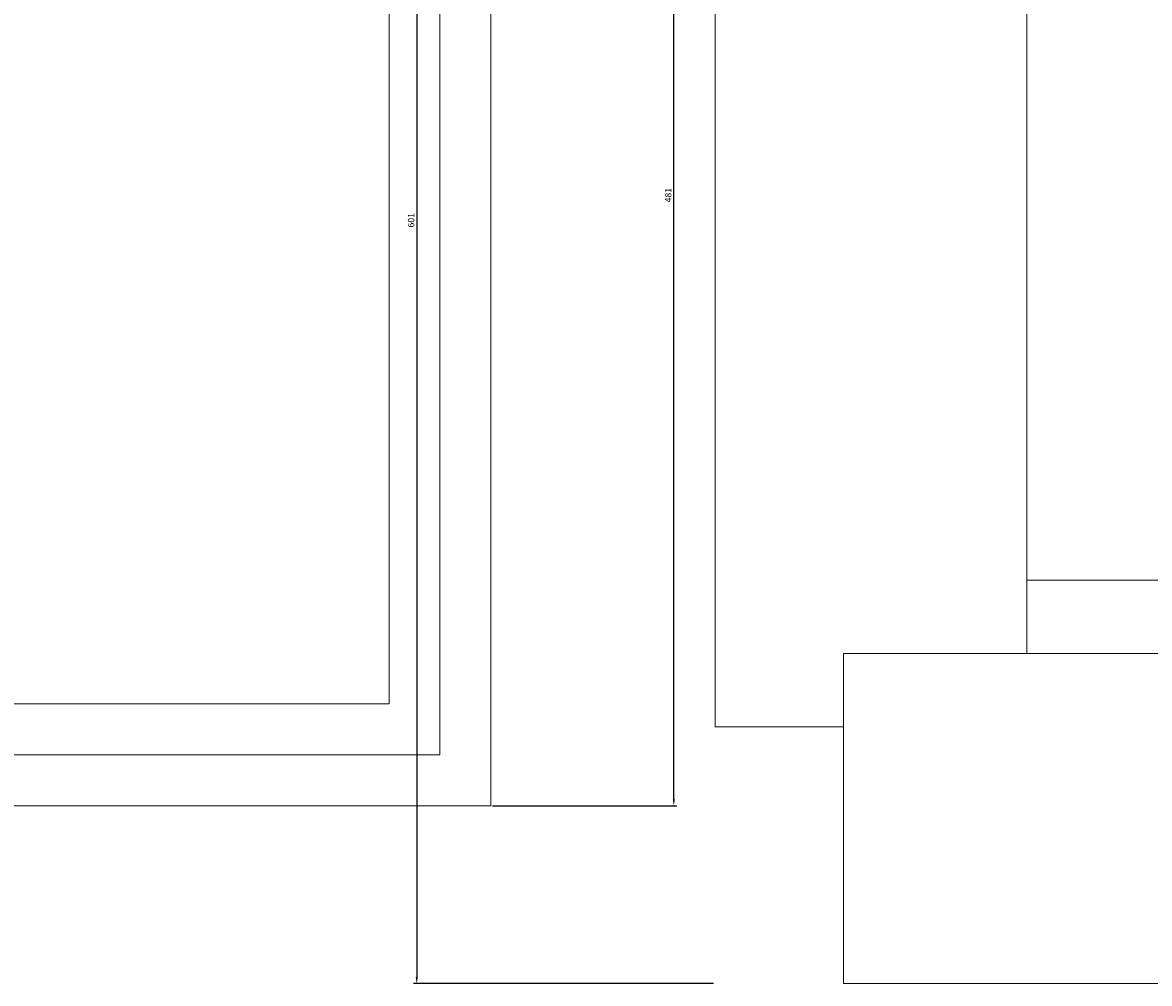
# Model space of a CAD drawing. Units: millimetres. Extents: x -857 to 54106, y -13666 to 13947.
# Tile 6 of 41: x 7861 to 8305, y 6233 to 6612. Entities that reach past the tile are written whole.
import ezdxf

# ---------------------------------------------------------------- set-up
doc = ezdxf.new("R2010")
doc.units = ezdxf.units.MM
for name, color, linetype, lineweight in [('A-ANNO-DIMS', 2, 'Continuous', 18), ('A-FURN', 21, 'Continuous', 18), ('A-FURNITURE', 25, 'Continuous', 9)]:
    doc.layers.add(name, color=color, linetype=linetype, lineweight=lineweight)
doc.styles.get("Standard").update_dxf_attribs({"font": 'arial.ttf'})
doc.dimstyles.new('ISO-25', dxfattribs={"dimtxt": 2.5, "dimasz": 2.5, "dimexe": 1.25, "dimexo": 0.625, "dimtad": 1, "dimtxsty": 'Standard', "dimcen": 2.5, "dimadec": 0, "dimazin": 0, "dimtfac": 1, "dimtmove": 0, "dimatfit": 3, "dimfxl": 1, "dimarcsym": 0})

# ---------------------------------------------------------------- blocks, each defined once
blk = doc.blocks.new('A$C21FE29A1')
at = {"layer": 'A-FURNITURE'}
for points in [[(0, 0), (24, 0), (24, 24), (0, 24)], [(1, 1), (23, 1), (23, 23), (1, 23)], [(2, 2), (22, 2), (22, 22), (2, 22)]]:
    blk.add_lwpolyline(points, close=True, dxfattribs=at)
blk = doc.blocks.new('A$C47E27A62')
at = {"layer": 'A-FURNITURE'}
for p, q in [((17.041, 0), (-17.041, 0)), ((17.041, 0), (17.041, -6.486)), ((17.041, -5.045), (19.563, -5.045)), ((19.563, -5.045), (19.563, -26.997)), ((17.041, -6.486), (-17.041, -6.486)), ((13.437, -6.486), (13.437, -26.997)), ((13.437, -7.927), (-13.437, -7.927))]:
    blk.add_line(p, q, dxfattribs=at)
blk = doc.blocks.new('*D58')
at = {"layer": 'A-ANNO-DIMS', "color": 0, "lineweight": -2, "transparency": 16777216}
for p, q in [((8046.39, 6784.17), (8119.14, 6784.17)), ((8117.89, 6305.8), (8117.89, 6781.67)), ((8046.39, 6303.3), (8119.14, 6303.3))]:
    blk.add_line(p, q, dxfattribs=at)
at = {"layer": 'A-ANNO-DIMS', "color": 0, "transparency": 16777216}
for points in [[(8117.48, 6781.67), (8118.31, 6781.67), (8117.89, 6784.17)], [(8117.48, 6305.8), (8118.31, 6305.8), (8117.89, 6303.3)]]:
    blk.add_solid(points, dxfattribs=at)
at = {"layer": 'Defpoints', "color": 0, "transparency": 16777216}
for p in [(8045.76, 6784.17), (8117.89, 6784.17), (8045.76, 6303.3)]:
    blk.add_point(p, dxfattribs=at)
at = {"layer": 'A-ANNO-DIMS', "color": 0, "transparency": 16777216, "insert": (8115.99, 6543.74), "char_height": 2.5, "attachment_point": 5, "rotation": 90}
blk.add_mtext('481', dxfattribs=at)
blk = doc.blocks.new('*D60')
at = {"layer": 'A-ANNO-DIMS', "color": 0, "lineweight": -2, "transparency": 16777216}
for p, q in [((8133.57, 6834.4), (8015.35, 6834.4)), ((8016.6, 6831.9), (8016.6, 6235.81)), ((8133.57, 6233.31), (8015.35, 6233.31))]:
    blk.add_line(p, q, dxfattribs=at)
at = {"layer": 'A-ANNO-DIMS', "color": 0, "transparency": 16777216}
for points in [[(8016.19, 6831.9), (8017.02, 6831.9), (8016.6, 6834.4)], [(8016.19, 6235.81), (8017.02, 6235.81), (8016.6, 6233.31)]]:
    blk.add_solid(points, dxfattribs=at)
at = {"layer": 'Defpoints', "color": 0, "transparency": 16777216}
for p in [(8134.19, 6834.4), (8016.6, 6233.31), (8134.19, 6233.31)]:
    blk.add_point(p, dxfattribs=at)
at = {"layer": 'A-ANNO-DIMS', "color": 0, "transparency": 16777216, "insert": (8014.7, 6533.85), "char_height": 2.5, "attachment_point": 5, "rotation": 90}
blk.add_mtext('601', dxfattribs=at)

msp = doc.modelspace()

# ---------------------------------------------------------------- block references
at = {"layer": 'A-FURN', "ltscale": 4, "xscale": 20.03650789584363, "yscale": 20.03650789584363, "zscale": 20.03650789584363, "rotation": 180}
msp.add_blockref('A$C47E27A62', (8526.165, 6233.305), dxfattribs=at)
at = {"layer": 'A-FURN', "xscale": 20.03650789584554, "yscale": 20.03650789584554, "zscale": 20.03650789584554, "rotation": 89.99999999999999}
msp.add_blockref('A$C21FE29A1', (8045.76, 6303.297), dxfattribs=at)

# ---------------------------------------------------------------- dimensions: what is measured, and where the dimension line sits
at = {"layer": 'A-ANNO-DIMS'}
for base, p1, p2, angle, picture, middle in [((8016.602, 6233.305), (8134.194, 6834.4), (8134.194, 6233.305), 270, '*D60', (8014.701, 6533.853)), ((8117.892, 6784.175), (8045.761, 6303.298), (8045.761, 6784.175), 90, '*D58', (8115.991, 6543.737))]:
    dim = msp.add_linear_dim(base=base, p1=p1, p2=p2, angle=angle, dimstyle='ISO-25', override={"dimdec": 0, "dimrnd": 0, "dimzin": 0, "dimlunit": 2}, dxfattribs=at)
    dim.commit()
    dim.dimension.update_dxf_attribs({"geometry": picture, "text_midpoint": middle})

doc.saveas('drawing.dxf')
